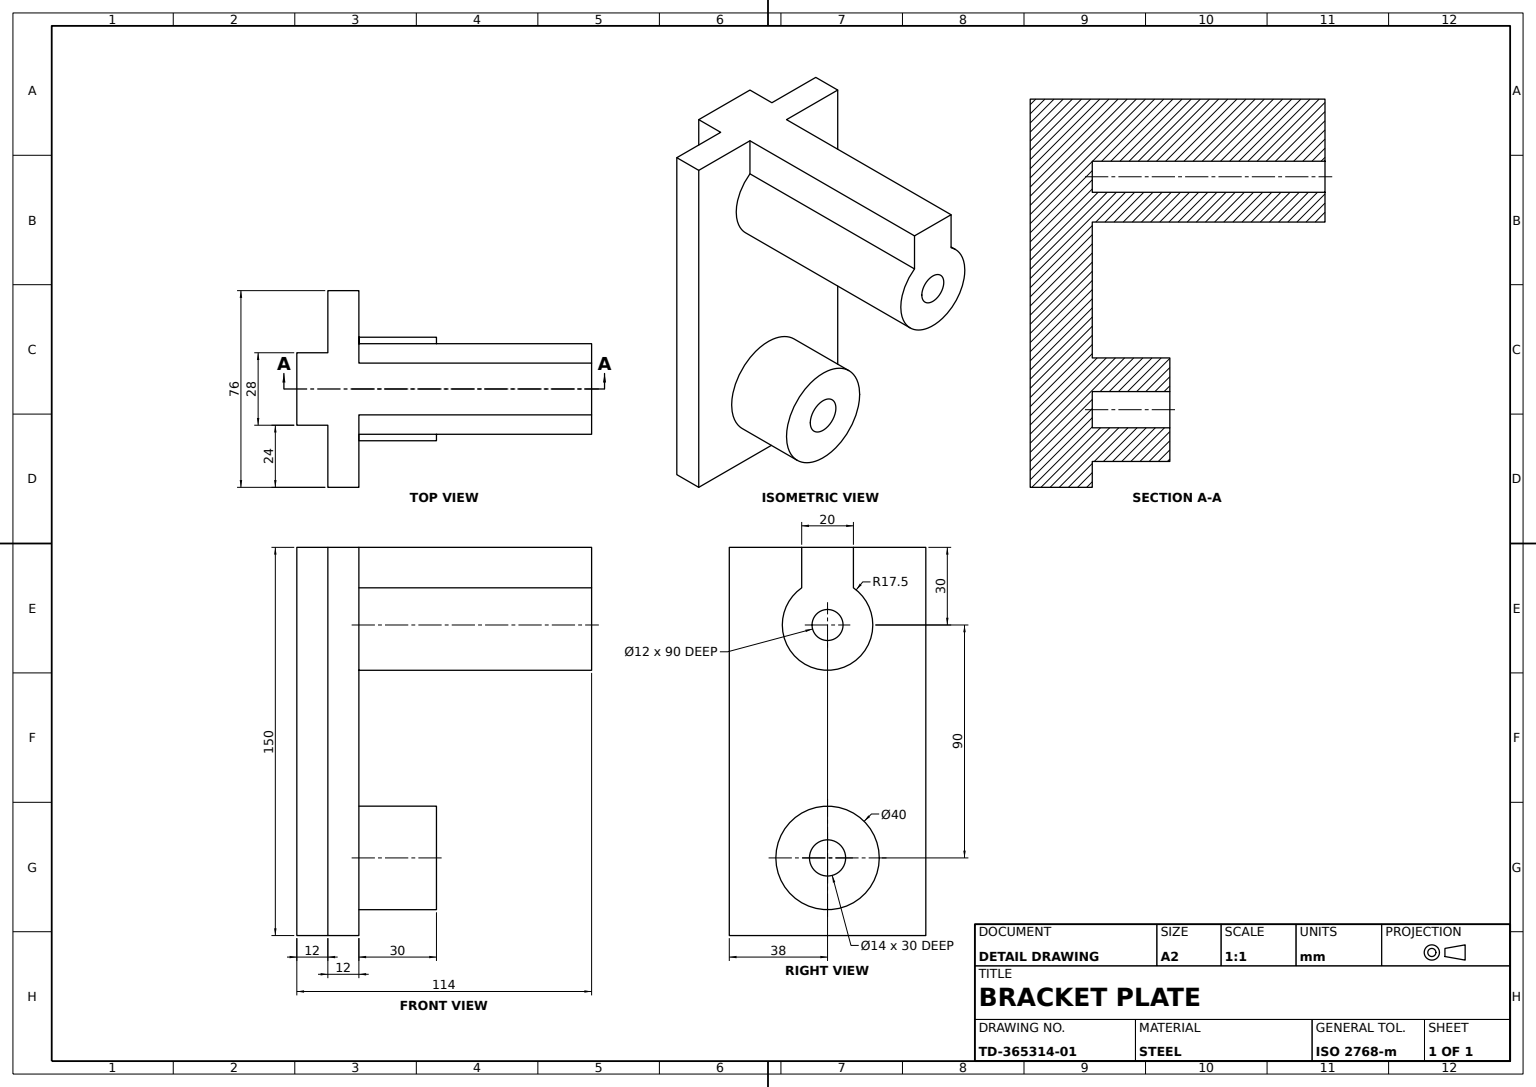
SolidWorks part; units mm, degrees
material "Plain Carbon Steel"
ref_plane "Front Plane" through (0, 0, 0) normal (0, 0, 1) x (1, 0, 0)
ref_plane "Top Plane" through (0, 0, 0) normal (0, 1, 0) x (1, 0, 0)
ref_plane "Right Plane" through (0, 0, 0) normal (1, 0, 0) x (0, 0, -1)
sketch "Base Plate Sketch" plane through (0, 0, 0) normal (0, 0, 1) x (1, 0, 0)
  line L1 (-38, -75) -> (38, -75)
  line L2 (-38, -75) -> (-38, 75)
  line L3 (-38, 75) -> (38, 75)
  line L4 (38, -75) -> (38, 75)
  line L5 (-38, -75) -> (38, 75) construction
  line L6 (-38, 75) -> (38, -75) construction
  point P0 (0, 0)
  dimension "D1" = 150
  dimension "D2" = 76
extrude "Base Plate" add sketch "Base Plate Sketch" along normal blind 12
sketch "Top Tab Sketch" plane through (0, -75, 0) normal (0, -1, 0) x (1, 0, 0)
  line L0 (-14, 0) -> (-14, -12)
  line L1 (-38, 0) -> (38, 0) construction
  line L2 (-14, -12) -> (14, -12)
  line L3 (14, -12) -> (14, 0)
  line L4 (-14, 0) -> (14, 0)
  dimension "D1" = 28
  dimension "D2" = 24
  dimension "D3" = 12
extrude "Top Tab" add sketch "Top Tab Sketch" against normal through all
sketch "Lower Bushing Boss Sketch" plane through (0, 0, 12) normal (0, 0, 1) x (1, 0, 0)
  line L0 (-38, -75) -> (38, -75) construction
  circle A0 centre (0, 45) radius 17.5
  circle A1 centre (0, -45) radius 20
  circle A2 centre (0, 45) radius 6
  circle A3 centre (0, -45) radius 7
  dimension "D3" = 40
  dimension "D4" = 35
  dimension "D5" = 12
  dimension "D6" = 14
  dimension "D1" = 30
  dimension "D2" = 90
extrude "Lower Bushing Boss" add sketch "Lower Bushing Boss Sketch" along normal blind 30 contours A1 A3
sketch "Upper Arm Sketch" plane through (0, 0, 12) normal (0, 0, 1) x (1, 0, 0)
  line L0 (38, 75) -> (-38, 75) construction
  circle A0 centre (0, 45) radius 17.5
  circle A1 centre (0, 45) radius 6
  dimension "D2" = 35
  dimension "D3" = 12
  dimension "D1" = 30
extrude "Upper Arm" add sketch "Upper Arm Sketch" along normal blind 90
sketch "Arm Rib Sketch" plane through (0, 75, 0) normal (0, 1, 0) x (1, 0, 0)
  line L0 (38, -12) -> (-38, -12) construction
  line L1 (-10, -12) -> (10, -12)
  line L2 (-10, -12) -> (-10, -102)
  line L3 (-10, -102) -> (10, -102)
  line L4 (10, -12) -> (10, -102)
  line L5 (-17.5, -102) -> (17.5, -102) construction
  point P8 (0, -12)
  dimension "D1" = 20
extrude "Arm Rib" add sketch "Arm Rib Sketch" against normal up to surface (15.6386 mm away)
